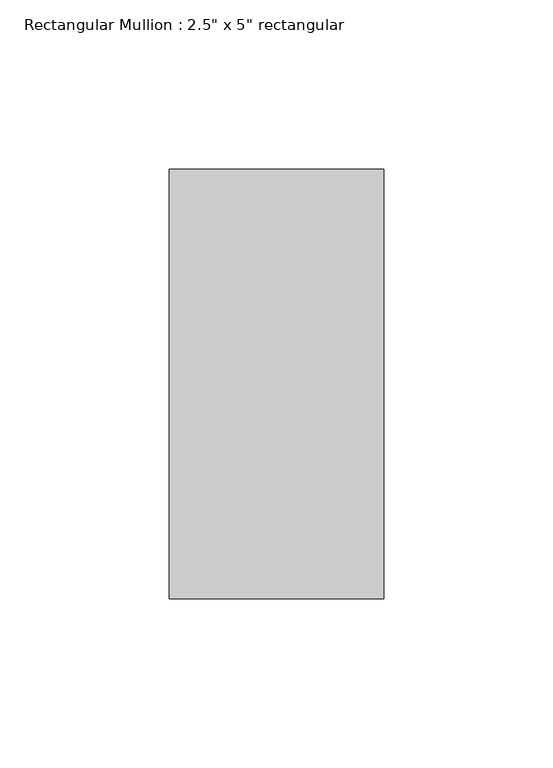
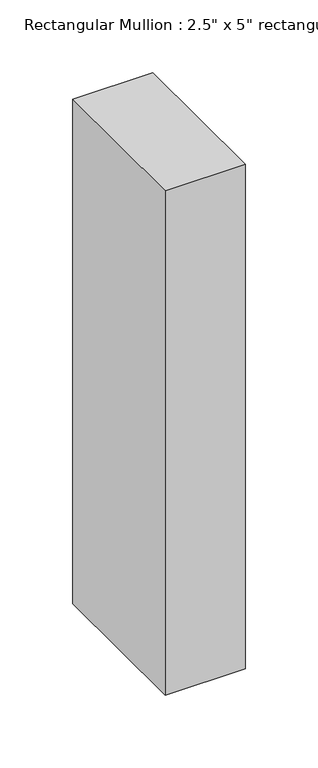
"""IFC4 building model written with IfcOpenShell, lengths in millimetres: member geometry."""

from ifc_helpers import new_model, si_unit, frame, origin, place, context, project, spatial, polyline, outline, extrude, source, transform, mapped, element, save


def member_6ea553f1(model_context):
    return source(origin(), model_context, "Body", "SweptSolid", [
        extrude(outline(polyline([(0.0, 63.5), (0.0, -63.5), (-63.5, -63.5), (-63.5, 63.5), (0.0, 63.5)])), frame((0.0, 0.0, -423.3333333), z_axis=(0.0, 0.0, 1.0), x_axis=(1.0, 0.0, 0.0)), (0.0, 0.0, 1.0), 423.3333333),
    ])


if __name__ == "__main__":
    model = new_model("IFC4")
    model_context = context("Model", 3, world=origin())
    ifc_project = project(units=[si_unit("LENGTHUNIT", "METRE", prefix="MILLI")], contexts=[model_context])
    site = spatial("IfcSite", under=ifc_project)
    building = spatial("IfcBuilding", under=site)
    placement = place(None, origin())
    member_shape = member_6ea553f1(model_context)
    element("IfcMember", 1, ObjectType="Rectangular Mullion : 2.5\" x 5\" rectangular", at=placement, inside=building, context=model_context, shape_type="MappedRepresentation", body=[
        mapped(member_shape, transform((0.0, 0.0, 0.0), x_axis=(1.0, 0.0, 0.0), y_axis=(0.0, 1.0, 0.0), z_axis=(0.0, 0.0, 1.0))),
    ])
    save(model, "model.ifc")

# Revit data of these elements
# Type "Rectangular Mullion : 2.5\" x 5\" rectangular"
#   built-in parameter 1007304 = 0.416667 (stored number, unit not read)
#   built-in parameter 1007301 = 0.104167 (stored number, unit not read)
#   built-in parameter 1007300 = 0.104167 (stored number, unit not read)
